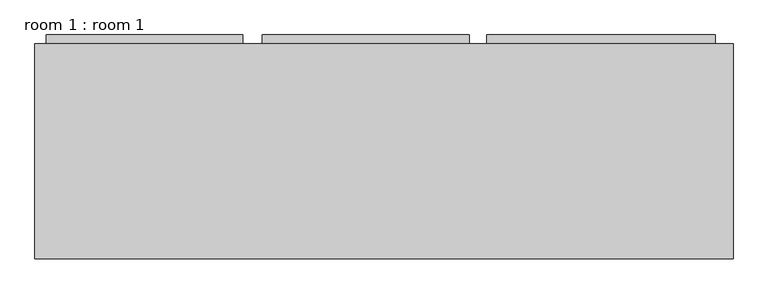
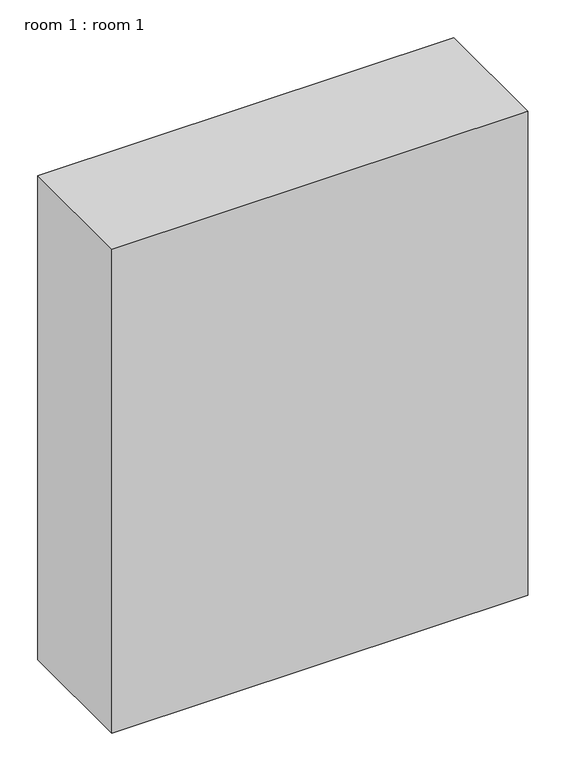
"""IFC4 building model written with IfcOpenShell, lengths in millimetres: proxy geometry, room 1 : room 1."""

from ifc_helpers import new_model, si_unit, frame, origin, origin_with_axes, place, context, project, spatial, polyline, outline, extrude, source, transform, mapped, element, save


def room_1_room_1_fc48c56b(model_context):
    return source(origin(), model_context, "Body", "SweptSolid", [
        extrude(outline(polyline([(-4065.2005972, 3589.6870892), (-3417.5005972, 3589.6870892), (-3417.5005972, 3564.2870892), (-4065.2005972, 3564.2870892), (-4065.2005972, 3589.6870892)])), frame((0.0, 0.0, 50.8), z_axis=(0.0, 0.0, 1.0), x_axis=(1.0, 0.0, 0.0)), (0.0, 0.0, 1.0), 2336.8),
        extrude(outline(polyline([(-4702.3537034, 3589.6870892), (-4116.0005972, 3589.6870892), (-4116.0005972, 3564.2870892), (-4702.3537034, 3564.2870892), (-4702.3537034, 3589.6870892)])), frame((0.0, 0.0, 50.8), z_axis=(0.0, 0.0, 1.0), x_axis=(1.0, 0.0, 0.0)), (0.0, 0.0, 1.0), 2336.8),
        extrude(outline(polyline([(-5315.7225796, 3589.6870892), (-4758.1493224, 3589.6870892), (-4758.1493224, 3564.2870892), (-5315.7225796, 3564.2870892), (-5315.7225796, 3589.6870892)])), frame((0.0, 0.0, 50.8), z_axis=(0.0, 0.0, 1.0), x_axis=(1.0, 0.0, 0.0)), (0.0, 0.0, 1.0), 2336.8),
        extrude(outline(polyline([(-3366.7005972, 2954.6870892), (-5347.9005972, 2954.6870892), (-5347.9005972, 3564.2870892), (-3366.7005972, 3564.2870892), (-3366.7005972, 2954.6870892)])), origin_with_axes(), (0.0, 0.0, 1.0), 2438.4),
    ])


if __name__ == "__main__":
    model = new_model("IFC4")
    model_context = context("Model", 3, world=origin())
    ifc_project = project(units=[si_unit("LENGTHUNIT", "METRE", prefix="MILLI")], contexts=[model_context])
    site = spatial("IfcSite", under=ifc_project)
    building = spatial("IfcBuilding", under=site)
    placement = place(None, origin())
    room_1_room_1_shape = room_1_room_1_fc48c56b(model_context)
    element("IfcBuildingElementProxy", 1, Name="room 1 : room 1", ObjectType="room 1 : room 1", at=placement, inside=building, context=model_context, shape_type="MappedRepresentation", body=[
        mapped(room_1_room_1_shape, transform((0.0, 0.0, 0.0), x_axis=(1.0, 0.0, 0.0), y_axis=(0.0, 1.0, 0.0), z_axis=(0.0, 0.0, 1.0))),
    ])
    save(model, "model.ifc")

# Revit data of these elements
# Element 1 (IfcBuildingElementProxy, "room 1 : room 1")
#   Materials on its faces: "Door - Frame/Mullion", "Door - Panel"
# Materials
#   "Door - Frame/Mullion": class "Wood", colour RGB 212 179 113, transparency 0
#   "Door - Panel": class "Wood", colour RGB 210 159 95, transparency 0, Cost = 0
